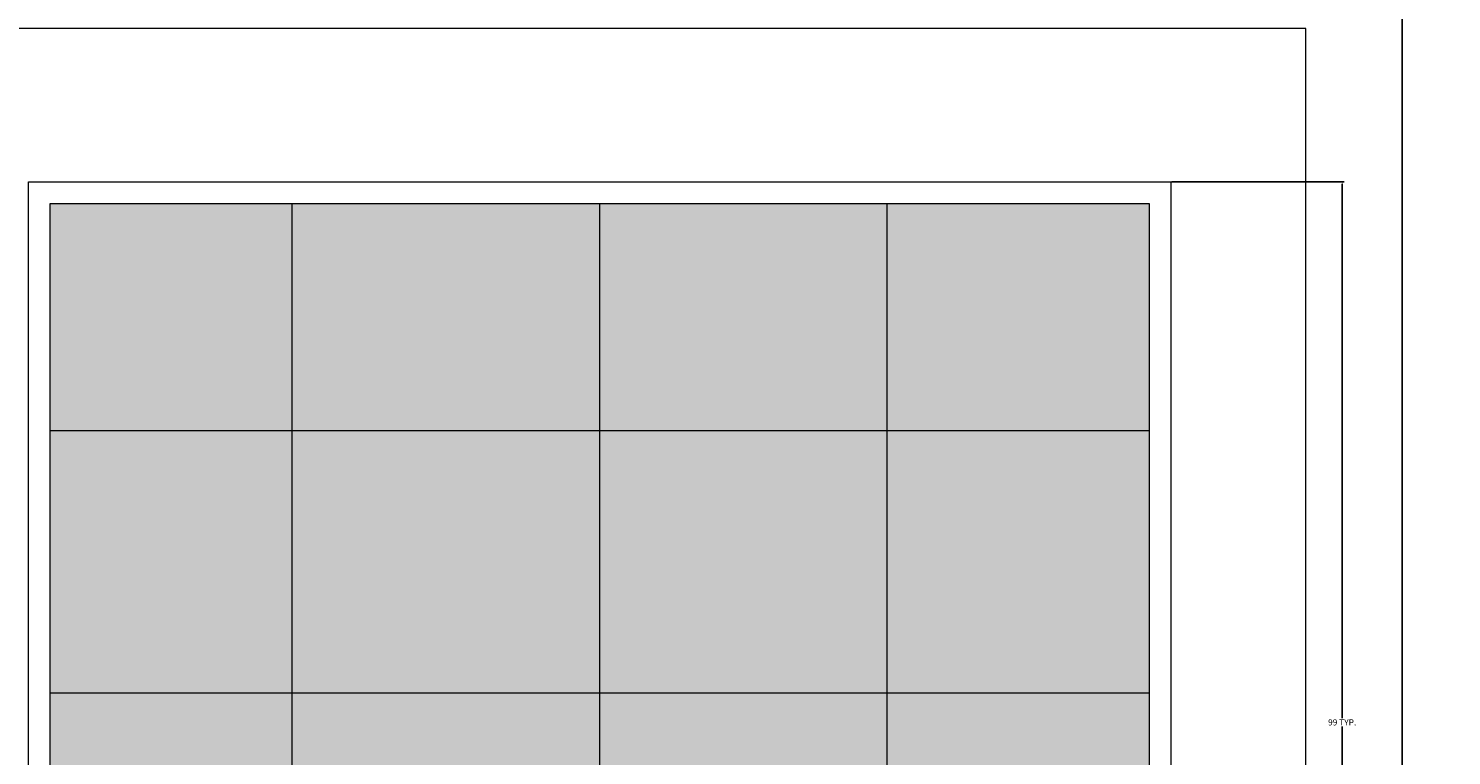
# Model space of a CAD drawing. Units: inches. Extents: x -26 to 776, y -22 to 650.
# Tile 13 of 62: x 92 to 222, y 353 to 420. Entities that reach past the tile are written whole.
import ezdxf

# ---------------------------------------------------------------- set-up
doc = ezdxf.new("R2010")
doc.units = ezdxf.units.IN
doc.header["$MEASUREMENT"] = 0
for name, color, linetype, lineweight in [('A-ANNO-DIMS', 2, 'Continuous', 18), ('A-GLAZ', 4, 'Continuous', 18), ('A-GLAZ-PATT', 9, 'Continuous', 13), ('A-WALL-TRIM', 7, 'Continuous', 18)]:
    doc.layers.add(name, color=color, linetype=linetype, lineweight=lineweight)
doc.styles.get("Standard").update_dxf_attribs({"font": 'arial.ttf'})
doc.dimstyles.get("Standard").update_dxf_attribs({"dimtxt": 0.5625, "dimasz": 0.18, "dimexe": 0.18, "dimexo": 0.0625, "dimgap": 0.09, "dimtad": 0, "dimtih": 1, "dimtoh": 1, "dimdec": 4, "dimzin": 0, "dimdsep": 46, "dimlunit": 4, "dimtxsty": 'Standard', "dimcen": 0.09, "dimadec": 0, "dimazin": 0, "dimtfac": 1, "dimtdec": 4, "dimtofl": 0, "dimtmove": 0, "dimatfit": 3, "dimfxl": 1, "dimtolj": 1, "dimtzin": 0, "dimarcsym": 0})

# ---------------------------------------------------------------- blocks, each defined once
blk = doc.blocks.new('WIN-ELEV-4X4')
for p, q in [((24.2, 97.34), (24.2, 2)), ((52.51, 97.34), (52.51, 2)), ((78.9, 97.34), (78.9, 2)), ((2, 76.47), (103.02, 76.47)), ((2, 76.47), (103.02, 76.47)), ((2, 52.37), (103.02, 52.37)), ((2, 26.9), (103.02, 26.9))]:
    blk.add_line(p, q)
for points in [[(0, 99.34), (105.02, 99.34), (105.02, 0), (0, 0)], [(2, 97.34), (103.02, 97.34), (103.02, 2), (2, 2)]]:
    blk.add_lwpolyline(points, close=True)
blk = doc.blocks.new('*D8')
at = {"layer": 'A-ANNO-DIMS', "color": 0, "lineweight": -2, "transparency": 16777216}
for p, q in [((196.73, 406.19), (212.6, 406.19)), ((212.42, 406.01), (212.42, 356.9)), ((212.42, 307.04), (212.42, 356.15)), ((196.73, 306.86), (212.6, 306.86))]:
    blk.add_line(p, q, dxfattribs=at)
at = {"layer": 'A-ANNO-DIMS', "color": 0, "transparency": 16777216}
for points in [[(212.39, 406.01), (212.45, 406.01), (212.42, 406.19)], [(212.39, 307.04), (212.45, 307.04), (212.42, 306.86)]]:
    blk.add_solid(points, dxfattribs=at)
at = {"layer": 'Defpoints', "color": 0, "transparency": 16777216}
for p in [(196.67, 406.19), (212.42, 406.19), (196.67, 306.86)]:
    blk.add_point(p, dxfattribs=at)
at = {"layer": 'A-ANNO-DIMS', "color": 0, "transparency": 16777216, "insert": (212.42, 356.52), "char_height": 0.5625, "attachment_point": 5}
blk.add_mtext('\\A1;99 TYP.', dxfattribs=at)
blk = doc.blocks.new('*D14')
at = {"layer": 'A-ANNO-DIMS', "color": 0, "lineweight": -2, "transparency": 16777216}
for p, q in [((191.62, 613.27), (-25.48, 613.27)), ((-25.3, 613.09), (-25.3, 314.75)), ((-25.3, 15.66), (-25.3, 314)), ((11.04, 15.48), (-25.48, 15.48))]:
    blk.add_line(p, q, dxfattribs=at)
at = {"layer": 'A-ANNO-DIMS', "color": 0, "transparency": 16777216}
for points in [[(-25.33, 613.09), (-25.27, 613.09), (-25.3, 613.27)], [(-25.33, 15.66), (-25.27, 15.66), (-25.3, 15.48)]]:
    blk.add_solid(points, dxfattribs=at)
at = {"layer": 'Defpoints', "color": 0, "transparency": 16777216}
for p in [(-25.3, 613.27), (191.68, 613.27), (11.11, 15.48)]:
    blk.add_point(p, dxfattribs=at)
at = {"layer": 'A-ANNO-DIMS', "color": 0, "transparency": 16777216, "insert": (-25.3, 314.38), "char_height": 0.562, "attachment_point": 5}
blk.add_mtext('\\A1;597.8', dxfattribs=at)
blk = doc.blocks.new('*D22')
at = {"layer": 'A-ANNO-DIMS', "color": 0, "lineweight": -2, "transparency": 16777216}
for p, q in [((22.89, 15.33), (22.89, 649.86)), ((23.07, 649.68), (119.19, 649.68)), ((217.77, 649.68), (121.65, 649.68)), ((217.95, 15.54), (217.95, 649.86))]:
    blk.add_line(p, q, dxfattribs=at)
at = {"layer": 'A-ANNO-DIMS', "color": 0, "transparency": 16777216}
for points in [[(23.07, 649.71), (23.07, 649.65), (22.89, 649.68)], [(217.77, 649.71), (217.77, 649.65), (217.95, 649.68)]]:
    blk.add_solid(points, dxfattribs=at)
at = {"layer": 'Defpoints', "color": 0, "transparency": 16777216}
for p in [(217.95, 649.68), (22.89, 15.27), (217.95, 15.48)]:
    blk.add_point(p, dxfattribs=at)
at = {"layer": 'A-ANNO-DIMS', "color": 0, "transparency": 16777216, "insert": (120.42, 649.68), "char_height": 0.562, "attachment_point": 5}
blk.add_mtext('\\A1;195.06', dxfattribs=at)

msp = doc.modelspace()

# ---------------------------------------------------------------- hatches: boundary and pattern name
at = {"layer": 'A-GLAZ-PATT'}
h = msp.add_hatch(dxfattribs=at)
h.set_pattern_fill('GOST_GLASS', color=256, scale=0.75)
h.set_pattern_definition([(45, (0, 0), (6.36396, 0), [3.75, -5.25]), (45, (1.591, 0), (6.36396, 0), [1.5, -7.5]), (45, (0, 1.591), (6.36396, 0), [1.5, -7.5])])
h.paths.add_polyline_path([(115.8402, 198.8773), (93.6448, 198.8773), (93.6448, 173.9734), (115.8402, 173.9734)])
h.paths.add_polyline_path([(144.1571, 198.8773), (115.8402, 198.8773), (115.8402, 173.9734), (144.1571, 173.9734)])
h.paths.add_polyline_path([(115.8402, 224.3396), (93.6448, 224.3396), (93.6448, 198.8773), (115.8402, 198.8773)])
h.paths.add_polyline_path([(144.1571, 248.4417), (115.8402, 248.4417), (115.8402, 224.3396), (144.1571, 224.3396)])
h.paths.add_polyline_path([(144.1571, 224.3396), (115.8402, 224.3396), (115.8402, 198.8773), (144.1571, 198.8773)])
h.paths.add_polyline_path([(170.5449, 224.3396), (144.1571, 224.3396), (144.1571, 198.8773), (170.5449, 198.8773)])
h.paths.add_polyline_path([(170.5449, 198.8773), (144.1571, 198.8773), (144.1571, 173.9734), (170.5449, 173.9734)])
h.paths.add_polyline_path([(194.6694, 198.8773), (170.5449, 198.8773), (170.5449, 173.9734), (194.6694, 173.9734)])
h.paths.add_polyline_path([(194.6694, 224.3396), (170.5449, 224.3396), (170.5449, 198.8773), (194.6694, 198.8773)])
h.paths.add_polyline_path([(194.6694, 248.4417), (170.5449, 248.4417), (170.5449, 224.3396), (194.6694, 224.3396)])
h.paths.add_polyline_path([(170.5449, 248.4417), (144.1571, 248.4417), (144.1571, 224.3396), (170.5449, 224.3396)])
h.paths.add_polyline_path([(144.1571, 269.3091), (115.8402, 269.3091), (115.8402, 248.4417), (144.1571, 248.4417)])
h.paths.add_polyline_path([(115.8402, 269.3091), (93.6448, 269.3091), (93.6448, 248.4417), (115.8402, 248.4417)])
h.paths.add_polyline_path([(115.8402, 248.4417), (93.6448, 248.4417), (93.6448, 224.3396), (115.8402, 224.3396)])
h.paths.add_polyline_path([(170.5449, 269.3091), (144.1571, 269.3091), (144.1571, 248.4417), (170.5449, 248.4417)])
h.paths.add_polyline_path([(194.6694, 269.3091), (170.5449, 269.3091), (170.5449, 248.4417), (194.6694, 248.4417)])
h.paths.add_polyline_path([(259.7413, 294.4171), (236.4647, 294.4171), (236.4647, 266.1888), (259.7413, 266.1888)])
h.paths.add_polyline_path([(285.0179, 294.4171), (261.7413, 294.4171), (261.7413, 266.1888), (285.0179, 266.1888)])
h.paths.add_polyline_path([(285.0179, 265.1888), (261.7413, 265.1888), (261.7413, 233.9172), (285.0179, 233.9172)])
h.paths.add_polyline_path([(259.7413, 265.1888), (236.4647, 265.1888), (236.4647, 233.9172), (259.7413, 233.9172)])
h.paths.add_polyline_path([(259.7413, 232.9172), (236.4647, 232.9172), (236.4647, 207.1741), (259.7413, 207.1741)])
h.paths.add_polyline_path([(285.0179, 232.9172), (261.7413, 232.9172), (261.7413, 207.1741), (285.0179, 207.1741)])
h.paths.add_polyline_path([(285.0179, 206.1741), (261.7413, 206.1741), (261.7413, 199.3298), (278.1134, 199.3298), (278.1134, 171.4173), (285.0179, 171.4173)])
h.paths.add_polyline_path([(259.7413, 206.1741), (236.4647, 206.1741), (236.4647, 199.3298), (259.7413, 199.3298)])
h.paths.add_polyline_path([(259.7413, 197.3298), (236.4647, 197.3298), (236.4647, 171.4173), (259.7413, 171.4173)])
h.paths.add_polyline_path([(276.1134, 197.3298), (261.7413, 197.3298), (261.7413, 171.4173), (276.1134, 171.4173)], flags=17)
h.paths.add_polyline_path([(255.8125, 548.0348), (228.5733, 548.0348), (228.5733, 528.3585), (255.8125, 528.3585)])
h.paths.add_polyline_path([(281.6181, 548.0348), (256.0792, 548.0348), (256.0792, 528.3585), (281.6181, 528.3585)])
h.paths.add_polyline_path([(308.8797, 548.0348), (281.789, 548.0348), (281.789, 528.3585), (308.8797, 528.3585)])
h.paths.add_polyline_path([(357.2724, 548.0995), (309.2457, 548.0348), (309.2457, 528.3585), (357.3034, 528.4233), (357.3034, 538.2614)])
h.paths.add_polyline_path([(259.7413, 437.1188), (236.4647, 437.1188), (236.4647, 408.8905), (259.7413, 408.8905)])
h.paths.add_polyline_path([(285.0179, 437.1188), (261.7413, 437.1188), (261.7413, 408.8905), (285.0179, 408.8905)])
h.paths.add_polyline_path([(259.7413, 407.8905), (236.4647, 407.8905), (236.4647, 376.6189), (259.7413, 376.6189)])
h.paths.add_polyline_path([(285.0179, 407.8905), (261.7413, 407.8905), (261.7413, 376.6189), (285.0179, 376.6189)])
h.paths.add_polyline_path([(285.0179, 375.6189), (261.7413, 375.6189), (261.7413, 349.8758), (285.0179, 349.8758)])
h.paths.add_polyline_path([(285.0179, 348.8758), (261.7413, 348.8758), (261.7413, 314.119), (285.0179, 314.119)])
h.paths.add_polyline_path([(259.7413, 348.8758), (236.4647, 348.8758), (236.4647, 314.119), (259.7413, 314.119)])
h.paths.add_polyline_path([(259.7413, 375.6189), (236.4647, 375.6189), (236.4647, 349.8758), (259.7413, 349.8758)])
h.paths.add_polyline_path([(194.6694, 404.1909), (170.5449, 404.1909), (170.5449, 383.3235), (194.6694, 383.3235)])
h.paths.add_polyline_path([(170.5449, 404.1909), (144.1571, 404.1909), (144.1571, 383.3235), (170.5449, 383.3235)])
h.paths.add_polyline_path([(144.1571, 404.1909), (115.8402, 404.1909), (115.8402, 383.3235), (144.1571, 383.3235)])
h.paths.add_polyline_path([(115.8402, 404.1909), (93.6448, 404.1909), (93.6448, 383.3235), (115.8402, 383.3235)])
h.paths.add_polyline_path([(115.8402, 383.3235), (93.6448, 383.3235), (93.6448, 359.2214), (115.8402, 359.2214)])
h.paths.add_polyline_path([(144.1571, 383.3235), (115.8402, 383.3235), (115.8402, 359.2214), (144.1571, 359.2214)])
h.paths.add_polyline_path([(115.8402, 359.2214), (93.6448, 359.2214), (93.6448, 333.7591), (115.8402, 333.7591)])
h.paths.add_polyline_path([(144.1571, 359.2214), (115.8402, 359.2214), (115.8402, 333.7591), (144.1571, 333.7591)])
h.paths.add_polyline_path([(115.8402, 333.7591), (93.6448, 333.7591), (93.6448, 308.8552), (115.8402, 308.8552)])
h.paths.add_polyline_path([(144.1571, 333.7591), (115.8402, 333.7591), (115.8402, 308.8552), (144.1571, 308.8552)])
h.paths.add_polyline_path([(170.5449, 333.7591), (144.1571, 333.7591), (144.1571, 308.8552), (170.5449, 308.8552)])
h.paths.add_polyline_path([(170.5449, 359.2214), (144.1571, 359.2214), (144.1571, 333.7591), (170.5449, 333.7591)])
h.paths.add_polyline_path([(170.5449, 383.3235), (144.1571, 383.3235), (144.1571, 359.2214), (170.5449, 359.2214)])
h.paths.add_polyline_path([(194.6694, 383.3235), (170.5449, 383.3235), (170.5449, 359.2214), (194.6694, 359.2214)])
h.paths.add_polyline_path([(194.6694, 359.2214), (170.5449, 359.2214), (170.5449, 333.7591), (194.6694, 333.7591)])
h.paths.add_polyline_path([(194.6694, 333.7591), (170.5449, 333.7591), (170.5449, 308.8552), (194.6694, 308.8552)])

# ---------------------------------------------------------------- linework, layer by layer
at = {"layer": 'A-WALL-TRIM'}
msp.add_lwpolyline([(82.134, 159.4824), (209.091, 159.4824), (209.091, 420.2783), (82.134, 420.2783)], close=True, dxfattribs=at)

# ---------------------------------------------------------------- block references
at = {"layer": 'A-GLAZ'}
msp.add_blockref('WIN-ELEV-4X4', (91.645, 306.855), dxfattribs=at)

# ---------------------------------------------------------------- dimensions: what is measured, and where the dimension line sits
at = {"layer": 'A-ANNO-DIMS'}
dim = msp.add_linear_dim(base=(217.9529, 649.6763), p1=(22.8891, 15.2701), p2=(217.9529, 15.4824), dimstyle='Standard', override={"dimdec": 2, "dimlfac": 1, "dimrnd": 0, "dimzin": 0, "dimdsep": 46, "dimlunit": 2}, dxfattribs=at)
dim.commit()
dim.dimension.update_dxf_attribs({"geometry": '*D22', "text_midpoint": (120.421, 649.6763)})
dim = msp.add_linear_dim(base=(-25.2976, 613.2713), p1=(11.1074, 15.4824), p2=(191.6782, 613.2713), angle=90, dimstyle='Standard', override={"dimdec": 1, "dimlfac": 1, "dimrnd": 0, "dimzin": 0, "dimdsep": 46, "dimlunit": 2}, dxfattribs=at)
dim.commit()
dim.dimension.update_dxf_attribs({"geometry": '*D14', "text_midpoint": (-25.2976, 314.3769)})
dim = msp.add_linear_dim(base=(212.4231, 406.1909), p1=(196.6694, 306.8552), p2=(196.6694, 406.1909), angle=90, text='<> TYP.', dimstyle='Standard', override={"dimdec": 0, "dimlfac": 1, "dimrnd": 0, "dimzin": 0, "dimdsep": 46, "dimlunit": 2}, dxfattribs=at)
dim.commit()
dim.dimension.update_dxf_attribs({"geometry": '*D8', "text_midpoint": (212.4231, 356.523)})

doc.saveas('drawing.dxf')
